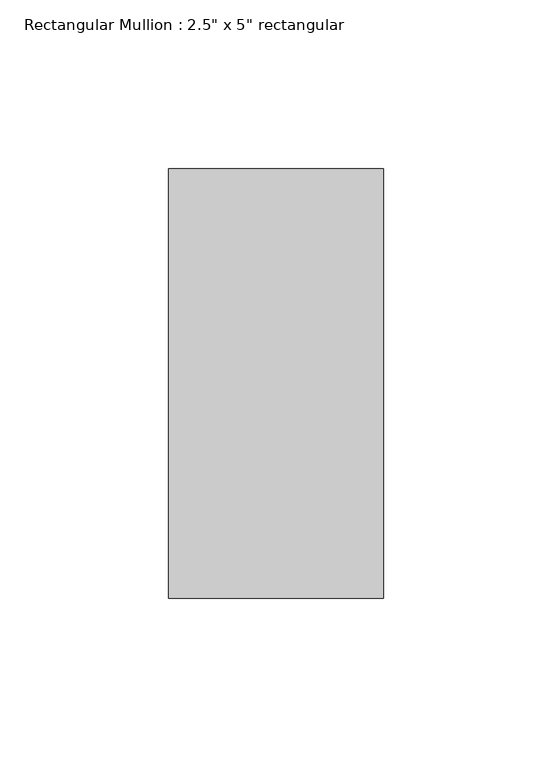
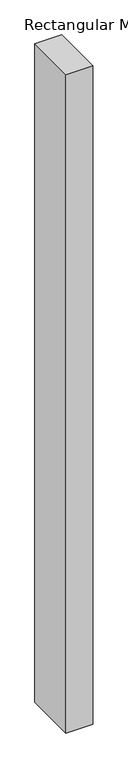
"""IFC4 building model written with IfcOpenShell, lengths in millimetres: member geometry."""

from ifc_helpers import new_model, si_unit, frame, origin, place, context, project, spatial, polyline, outline, extrude, source, transform, mapped, element, save


def member_28ac88d2(model_context):
    return source(origin(), model_context, "Body", "SweptSolid", [
        extrude(outline(polyline([(31.75, 63.5), (31.75, -63.5), (-31.75, -63.5), (-31.75, 63.5), (31.75, 63.5)])), frame((0.0, 0.0, -1649.9537661), z_axis=(0.0, 0.0, 1.0), x_axis=(1.0, 0.0, 0.0)), (0.0, 0.0, 1.0), 1649.9537661),
    ])


if __name__ == "__main__":
    model = new_model("IFC4")
    model_context = context("Model", 3, world=origin())
    ifc_project = project(units=[si_unit("LENGTHUNIT", "METRE", prefix="MILLI")], contexts=[model_context])
    site = spatial("IfcSite", under=ifc_project)
    building = spatial("IfcBuilding", under=site)
    placement = place(None, origin())
    member_shape = member_28ac88d2(model_context)
    element("IfcMember", 1, ObjectType="Rectangular Mullion : 2.5\" x 5\" rectangular", at=placement, inside=building, context=model_context, shape_type="MappedRepresentation", body=[
        mapped(member_shape, transform((0.0, 0.0, 0.0), x_axis=(1.0, 0.0, 0.0), y_axis=(0.0, 1.0, 0.0), z_axis=(0.0, 0.0, 1.0))),
    ])
    save(model, "model.ifc")

# Revit data of these elements
# Type "Rectangular Mullion : 2.5\" x 5\" rectangular"
#   built-in parameter 1007304 = 0.416667 (stored number, unit not read)
#   built-in parameter 1007301 = 0.104167 (stored number, unit not read)
#   built-in parameter 1007300 = 0.104167 (stored number, unit not read)
# Element 1 (IfcMember, "Rectangular Mullion : 2.5\" x 5\" rectangular")
#   Materials on its faces: "Aluminum"
# Materials
#   "Aluminum": class "Metal", colour RGB 247 247 247, transparency 0, Description = "Aluminum 6061", Cost = 0
